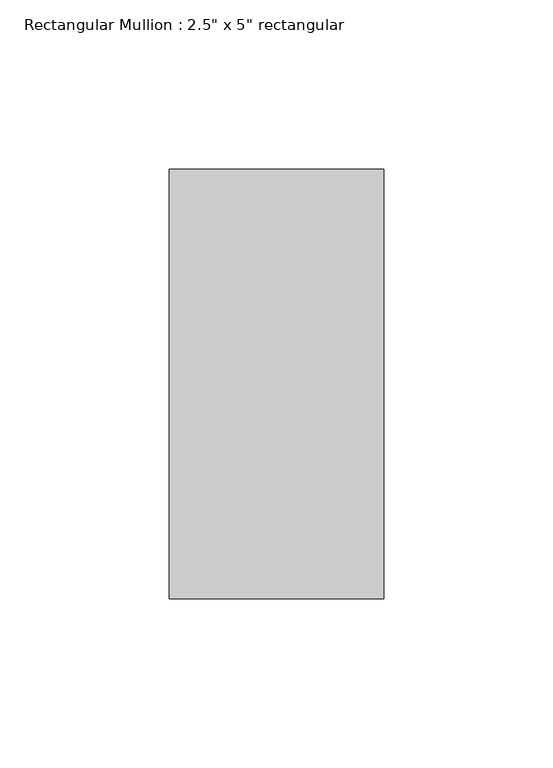
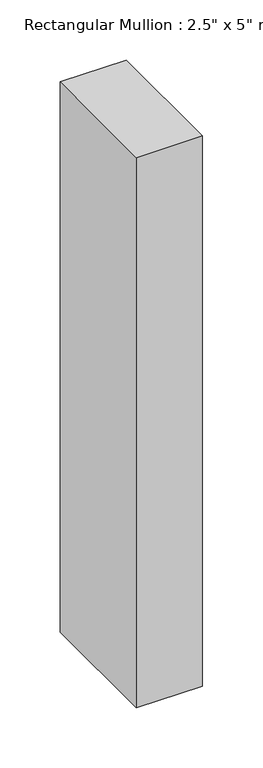
"""IFC4 building model written with IfcOpenShell, lengths in millimetres: member geometry."""

from ifc_helpers import new_model, si_unit, frame, origin, place, context, project, spatial, polyline, outline, extrude, source, transform, mapped, element, save


def member_bc554fa6(model_context):
    return source(origin(), model_context, "Body", "SweptSolid", [
        extrude(outline(polyline([(31.75, 63.5), (31.75, -63.5), (-31.75, -63.5), (-31.75, 63.5), (31.75, 63.5)])), frame((0.0, 0.0, -558.8), z_axis=(0.0, 0.0, 1.0), x_axis=(1.0, 0.0, 0.0)), (0.0, 0.0, 1.0), 558.8),
    ])


if __name__ == "__main__":
    model = new_model("IFC4")
    model_context = context("Model", 3, world=origin())
    ifc_project = project(units=[si_unit("LENGTHUNIT", "METRE", prefix="MILLI")], contexts=[model_context])
    site = spatial("IfcSite", under=ifc_project)
    building = spatial("IfcBuilding", under=site)
    placement = place(None, origin())
    member_shape = member_bc554fa6(model_context)
    element("IfcMember", 1, ObjectType="Rectangular Mullion : 2.5\" x 5\" rectangular", at=placement, inside=building, context=model_context, shape_type="MappedRepresentation", body=[
        mapped(member_shape, transform((0.0, 0.0, 0.0), x_axis=(1.0, 0.0, 0.0), y_axis=(0.0, 1.0, 0.0), z_axis=(0.0, 0.0, 1.0))),
    ])
    save(model, "model.ifc")

# Revit data of these elements
# Type "Rectangular Mullion : 2.5\" x 5\" rectangular"
#   built-in parameter 1007304 = 0.416667 (stored number, unit not read)
#   built-in parameter 1007301 = 0.104167 (stored number, unit not read)
#   built-in parameter 1007300 = 0.104167 (stored number, unit not read)
